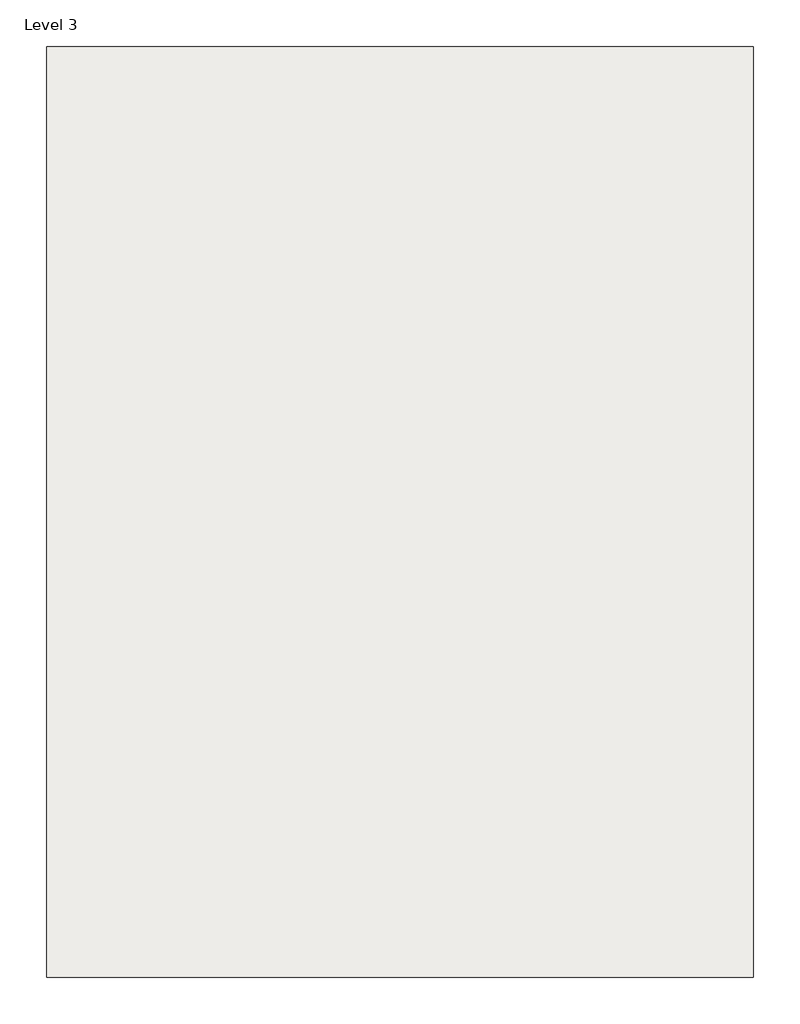
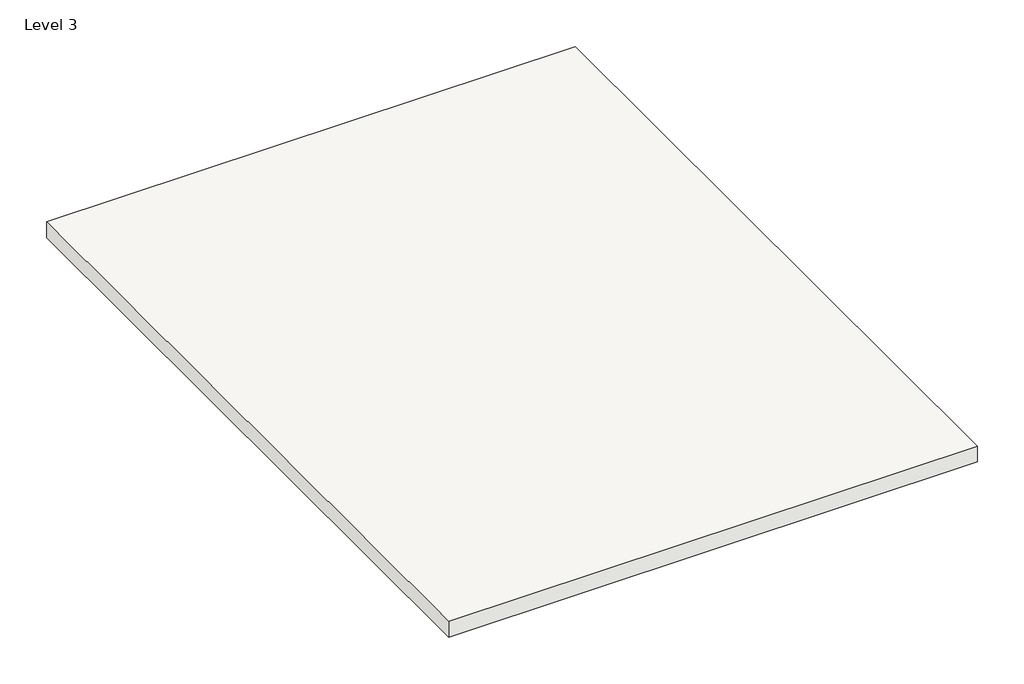
# One storey: 1 roof.
"""IFC4 building model written with IfcOpenShell, lengths in millimetres."""

from ifc_helpers import new_model, si_unit, frame, origin, place, context, project, spatial, polyline, outline, extrude, element, save

model = new_model("IFC4")

# Units and contexts
model_context = context("Model", 3, world=origin())
ifc_project = project(units=[si_unit("LENGTHUNIT", "METRE", prefix="MILLI")], contexts=[model_context])

# Site, building, storey
site = spatial("IfcSite", under=ifc_project)
building = spatial("IfcBuilding", under=site)
storey = spatial("IfcBuildingStorey", under=building, Name="Level 3", Elevation=6096.0)

# Roof
placement = place(None, origin())
element("IfcRoof", 1, ObjectType="Generic - 12\"", at=placement, inside=storey, context=model_context, shape_type="SweptSolid", body=[
    extrude(outline(polyline([(-15214.3530968, -317.658307), (-5613.1530968, -317.658307), (-5613.1530968, -12966.858307), (-15214.3530968, -12966.858307), (-15214.3530968, -317.658307)])), frame((0.0, 0.0, 6096.0), z_axis=(0.0, 0.0, 1.0), x_axis=(1.0, 0.0, 0.0)), (0.0, 0.0, 1.0), 304.8),
])

save(model, "model.ifc")

# Revit data of these elements
# Type "Generic - 12\""
#   Assembly Code = "B1020"
#   Layers, outside or top first: 1' - 0" no material (function 1)
# Element 1 (IfcRoof, "Generic - 12\"")
#   built-in parameter 1001705 = 21 (stored number, unit not read)
#   built-in parameter 1001710 = 33615
#   Phase Created = New Construction
#   Materials on its faces: "Default Roof"
# Materials
#   "Default Roof": colour RGB 88 101 114, transparency 0, Cost = 0
